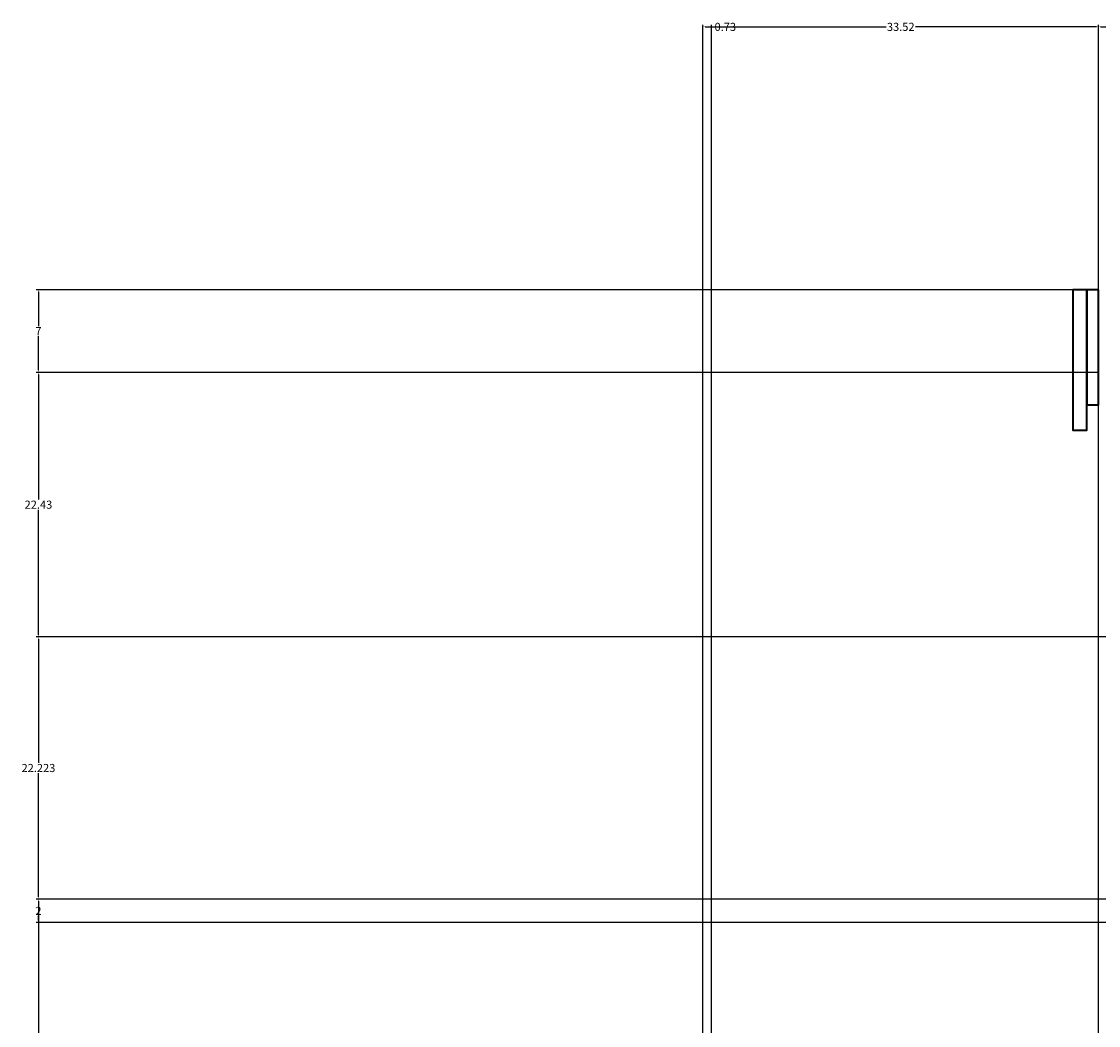
# Model space of a CAD drawing. Units: inches. Extents: x -139 to 346, y 72 to 413.
# Tile 6 of 18: x -139 to -47, y 328 to 413. Entities that reach past the tile are written whole.
import ezdxf

# ---------------------------------------------------------------- set-up
doc = ezdxf.new("R2010")
doc.units = ezdxf.units.IN
doc.header["$MEASUREMENT"] = 0
doc.layers.add('A-ANNO-DIMS', color=2, linetype='Continuous', lineweight=18)
doc.layers.add('A-ROOF', color=1, linetype='Continuous', lineweight=35)
doc.styles.get("Standard").update_dxf_attribs({"font": 'arial.ttf'})
doc.dimstyles.get("Standard").update_dxf_attribs({"dimtxt": 0.6875, "dimasz": 0.18, "dimexe": 0.18, "dimexo": 0.0625, "dimgap": 0.09, "dimtad": 0, "dimtih": 1, "dimtoh": 1, "dimdec": 4, "dimzin": 0, "dimdsep": 46, "dimlunit": 4, "dimtxsty": 'Standard', "dimcen": 0.09, "dimadec": 0, "dimazin": 0, "dimtfac": 1, "dimtdec": 4, "dimtofl": 0, "dimtmove": 0, "dimatfit": 3, "dimfxl": 1, "dimtolj": 1, "dimtzin": 0, "dimarcsym": 0})

# ---------------------------------------------------------------- blocks, each defined once
blk = doc.blocks.new('*D23')
at = {"layer": 'A-ANNO-DIMS', "color": 0, "lineweight": -2, "transparency": 16777216}
for p, q in [((-47.273, 383.037), (-47.273, 412.455)), ((-47.093, 412.275), (-22.053, 412.275)), ((5.493, 412.275), (-19.548, 412.275)), ((5.673, 338.384), (5.673, 412.455))]:
    blk.add_line(p, q, dxfattribs=at)
at = {"layer": 'A-ANNO-DIMS', "color": 0, "transparency": 16777216}
for points in [[(-47.093, 412.305), (-47.093, 412.245), (-47.273, 412.275)], [(5.493, 412.305), (5.493, 412.245), (5.673, 412.275)]]:
    blk.add_solid(points, dxfattribs=at)
at = {"layer": 'Defpoints', "color": 0, "transparency": 16777216}
for p in [(5.673, 412.275), (-47.273, 382.975), (5.673, 338.322)]:
    blk.add_point(p, dxfattribs=at)
at = {"layer": 'A-ANNO-DIMS', "color": 0, "transparency": 16777216, "insert": (-20.8, 412.275), "char_height": 0.6875, "attachment_point": 5}
blk.add_mtext('\\A1;52.95', dxfattribs=at)
blk = doc.blocks.new('*D44')
at = {"layer": 'A-ANNO-DIMS', "color": 0, "lineweight": -2, "transparency": 16777216}
for p, q in [((5.61, 338.322), (-137.304, 338.322)), ((-137.124, 338.142), (-137.124, 315.132)), ((-137.124, 291.24), (-137.124, 314.25)), ((-47.336, 291.06), (-137.304, 291.06))]:
    blk.add_line(p, q, dxfattribs=at)
at = {"layer": 'A-ANNO-DIMS', "color": 0, "transparency": 16777216}
for points in [[(-137.154, 338.142), (-137.094, 338.142), (-137.124, 338.322)], [(-137.154, 291.24), (-137.094, 291.24), (-137.124, 291.06)]]:
    blk.add_solid(points, dxfattribs=at)
at = {"layer": 'Defpoints', "color": 0, "transparency": 16777216}
for p in [(-137.124, 338.322), (5.673, 338.322), (-47.273, 291.06)]:
    blk.add_point(p, dxfattribs=at)
at = {"layer": 'A-ANNO-DIMS', "color": 0, "transparency": 16777216, "insert": (-137.124, 314.691), "char_height": 0.6875, "attachment_point": 5}
blk.add_mtext('\\A1;47.26', dxfattribs=at)
blk = doc.blocks.new('*D45')
at = {"layer": 'A-ANNO-DIMS', "color": 0, "lineweight": -2, "transparency": 16777216}
for p, q in [((-34.797, 360.544), (-137.304, 360.544)), ((-137.124, 360.364), (-137.124, 349.874)), ((-137.124, 338.502), (-137.124, 348.992)), ((5.61, 338.322), (-137.304, 338.322))]:
    blk.add_line(p, q, dxfattribs=at)
at = {"layer": 'A-ANNO-DIMS', "color": 0, "transparency": 16777216}
for points in [[(-137.154, 360.364), (-137.094, 360.364), (-137.124, 360.544)], [(-137.154, 338.502), (-137.094, 338.502), (-137.124, 338.322)]]:
    blk.add_solid(points, dxfattribs=at)
at = {"layer": 'Defpoints', "color": 0, "transparency": 16777216}
for p in [(-137.124, 360.544), (-34.735, 360.544), (5.673, 338.322)]:
    blk.add_point(p, dxfattribs=at)
at = {"layer": 'A-ANNO-DIMS', "color": 0, "transparency": 16777216, "insert": (-137.124, 349.433), "char_height": 0.6875, "attachment_point": 5}
blk.add_mtext('\\A1;22.223', dxfattribs=at)
blk = doc.blocks.new('*D46')
at = {"layer": 'A-ANNO-DIMS', "color": 0, "lineweight": -2, "transparency": 16777216}
for p, q in [((-47.336, 382.975), (-137.304, 382.975)), ((-137.124, 382.795), (-137.124, 372.201)), ((-137.124, 360.724), (-137.124, 371.318)), ((-34.797, 360.544), (-137.304, 360.544))]:
    blk.add_line(p, q, dxfattribs=at)
at = {"layer": 'A-ANNO-DIMS', "color": 0, "transparency": 16777216}
for points in [[(-137.154, 382.795), (-137.094, 382.795), (-137.124, 382.975)], [(-137.154, 360.724), (-137.094, 360.724), (-137.124, 360.544)]]:
    blk.add_solid(points, dxfattribs=at)
at = {"layer": 'Defpoints', "color": 0, "transparency": 16777216}
for p in [(-137.124, 382.975), (-47.273, 382.975), (-34.735, 360.544)]:
    blk.add_point(p, dxfattribs=at)
at = {"layer": 'A-ANNO-DIMS', "color": 0, "transparency": 16777216, "insert": (-137.124, 371.76), "char_height": 0.6875, "attachment_point": 5}
blk.add_mtext('\\A1;22.43', dxfattribs=at)
blk = doc.blocks.new('*D47')
at = {"layer": 'A-ANNO-DIMS', "color": 0, "lineweight": -2, "transparency": 16777216}
for p, q in [((-47.335936, 389.974785), (-137.303687, 389.974785)), ((-137.123687, 389.794785), (-137.123687, 386.908535)), ((-137.123687, 383.154785), (-137.123687, 386.041035)), ((-47.335936, 382.974785), (-137.303687, 382.974785))]:
    blk.add_line(p, q, dxfattribs=at)
at = {"layer": 'A-ANNO-DIMS', "color": 0, "transparency": 16777216}
for points in [[(-137.153687, 389.794785), (-137.093687, 389.794785), (-137.123687, 389.974785)], [(-137.153687, 383.154785), (-137.093687, 383.154785), (-137.123687, 382.974785)]]:
    blk.add_solid(points, dxfattribs=at)
at = {"layer": 'Defpoints', "color": 0, "transparency": 16777216}
for p in [(-137.123687, 389.974785), (-47.273436, 389.974785), (-47.273436, 382.974785)]:
    blk.add_point(p, dxfattribs=at)
at = {"layer": 'A-ANNO-DIMS', "color": 0, "transparency": 16777216, "insert": (-137.123687, 386.474785), "char_height": 0.6875, "attachment_point": 5}
blk.add_mtext('\\A1;7', dxfattribs=at)
blk = doc.blocks.new('*D49')
at = {"layer": 'A-ANNO-DIMS', "color": 0, "lineweight": -2, "transparency": 16777216}
for p, q in [((-80.796, 213.573), (-80.796, 412.455)), ((-80.616, 412.275), (-65.281, 412.275)), ((-47.453, 412.275), (-62.789, 412.275)), ((-47.273, 226.669), (-47.273, 412.455))]:
    blk.add_line(p, q, dxfattribs=at)
at = {"layer": 'A-ANNO-DIMS', "color": 0, "transparency": 16777216}
for points in [[(-80.616, 412.305), (-80.616, 412.245), (-80.796, 412.275)], [(-47.453, 412.305), (-47.453, 412.245), (-47.273, 412.275)]]:
    blk.add_solid(points, dxfattribs=at)
at = {"layer": 'Defpoints', "color": 0, "transparency": 16777216}
for p in [(-47.273, 412.275), (-47.273, 226.606), (-80.796, 213.511)]:
    blk.add_point(p, dxfattribs=at)
at = {"layer": 'A-ANNO-DIMS', "color": 0, "transparency": 16777216, "insert": (-64.035, 412.275), "char_height": 0.6875, "attachment_point": 5}
blk.add_mtext('\\A1;33.52', dxfattribs=at)
blk = doc.blocks.new('*D50')
at = {"layer": 'A-ANNO-DIMS', "color": 0, "lineweight": -2, "transparency": 16777216}
for p, q in [((-80.796, 213.573), (-80.796, 412.455)), ((-80.616, 412.275), (-80.248, 412.275)), ((-80.068, 211.71), (-80.068, 412.455)), ((-80.068, 412.275), (-79.888, 412.275))]:
    blk.add_line(p, q, dxfattribs=at)
at = {"layer": 'A-ANNO-DIMS', "color": 0, "transparency": 16777216}
for points in [[(-80.616, 412.305), (-80.616, 412.245), (-80.796, 412.275)], [(-80.248, 412.305), (-80.248, 412.245), (-80.068, 412.275)]]:
    blk.add_solid(points, dxfattribs=at)
at = {"layer": 'Defpoints', "color": 0, "transparency": 16777216}
for p in [(-80.068, 412.275), (-80.796, 213.511), (-80.068, 211.648)]:
    blk.add_point(p, dxfattribs=at)
at = {"layer": 'A-ANNO-DIMS', "color": 0, "transparency": 16777216, "insert": (-78.905, 412.275), "char_height": 0.6875, "attachment_point": 5}
blk.add_mtext('\\A1;0.73', dxfattribs=at)
blk = doc.blocks.new('*D89')
at = {"layer": 'A-ANNO-DIMS', "color": 0, "lineweight": -2, "transparency": 16777216}
for p, q in [((62.363, 338.322), (-137.304, 338.322)), ((-137.124, 338.142), (-137.124, 315.132)), ((-137.124, 291.24), (-137.124, 314.25)), ((62.363, 291.06), (-137.304, 291.06))]:
    blk.add_line(p, q, dxfattribs=at)
at = {"layer": 'A-ANNO-DIMS', "color": 0, "transparency": 16777216}
for points in [[(-137.154, 338.142), (-137.094, 338.142), (-137.124, 338.322)], [(-137.154, 291.24), (-137.094, 291.24), (-137.124, 291.06)]]:
    blk.add_solid(points, dxfattribs=at)
at = {"layer": 'Defpoints', "color": 0, "transparency": 16777216}
for p in [(-137.124, 338.322), (62.426, 338.322), (62.426, 291.06)]:
    blk.add_point(p, dxfattribs=at)
at = {"layer": 'A-ANNO-DIMS', "color": 0, "transparency": 16777216, "insert": (-137.124, 314.691), "char_height": 0.6875, "attachment_point": 5}
blk.add_mtext('\\A1;47.26', dxfattribs=at)
blk = doc.blocks.new('*D92')
at = {"layer": 'A-ANNO-DIMS', "color": 0, "lineweight": -2, "transparency": 16777216}
for p, q in [((62.363, 338.322), (-137.304, 338.322)), ((-137.124, 338.142), (-137.124, 337.757)), ((-137.124, 336.502), (-137.124, 336.887)), ((60.363, 336.322), (-137.304, 336.322))]:
    blk.add_line(p, q, dxfattribs=at)
at = {"layer": 'A-ANNO-DIMS', "color": 0, "transparency": 16777216}
for points in [[(-137.154, 338.142), (-137.094, 338.142), (-137.124, 338.322)], [(-137.154, 336.502), (-137.094, 336.502), (-137.124, 336.322)]]:
    blk.add_solid(points, dxfattribs=at)
at = {"layer": 'Defpoints', "color": 0, "transparency": 16777216}
for p in [(62.426, 338.322), (-137.124, 336.322), (60.426, 336.322)]:
    blk.add_point(p, dxfattribs=at)
at = {"layer": 'A-ANNO-DIMS', "color": 0, "transparency": 16777216, "insert": (-137.124, 337.322), "char_height": 0.6875, "attachment_point": 5}
blk.add_mtext('\\A1;2', dxfattribs=at)

msp = doc.modelspace()

# ---------------------------------------------------------------- linework, layer by layer
at = {"layer": 'A-ROOF'}
for points in [[(-48.2494, 389.9748), (-49.454, 389.9748), (-49.454, 378.0862), (-48.2494, 378.0862)], [(-47.2734, 389.9748), (-48.2494, 389.9748), (-48.2494, 380.2199), (-47.2734, 380.2199)]]:
    msp.add_lwpolyline(points, close=True, dxfattribs=at)

# ---------------------------------------------------------------- dimensions: what is measured, and where the dimension line sits
at = {"layer": 'A-ANNO-DIMS'}
for base, p1, p2, picture, middle in [((-47.2734, 412.2748), (-80.7961, 213.5107), (-47.2734, 226.6062), '*D49', (-64.0348, 412.2748)), ((-80.0684, 412.2748), (-80.7961, 213.5107), (-80.0684, 211.6478), '*D50', (-78.9055, 412.2748)), ((5.6729, 412.2748), (-47.2734, 382.9748), (5.6729, 338.3217), '*D23', (-20.8002, 412.2748))]:
    dim = msp.add_linear_dim(base=base, p1=p1, p2=p2, dimstyle='Standard', override={"dimdec": 2, "dimlfac": 1, "dimrnd": 0, "dimzin": 0, "dimdsep": 46, "dimlunit": 2}, dxfattribs=at)
    dim.commit()
    dim.dimension.update_dxf_attribs({"geometry": picture, "text_midpoint": middle})
for base, p1, p2, override, picture, middle in [((-137.1237, 389.9748), (-47.2734, 382.9748), (-47.2734, 389.9748), {"dimdec": 0, "dimlfac": 1, "dimrnd": 0, "dimzin": 0, "dimdsep": 46, "dimlunit": 2}, '*D47', (-137.1237, 386.4748)), ((-137.1237, 382.9748), (-34.7346, 360.5443), (-47.2734, 382.9748), {"dimdec": 2, "dimlfac": 1, "dimrnd": 0, "dimzin": 0, "dimdsep": 46, "dimlunit": 2}, '*D46', (-137.1237, 371.7595)), ((-137.1237, 360.5443), (5.6729, 338.3217), (-34.7346, 360.5443), {"dimdec": 3, "dimlfac": 1, "dimrnd": 0, "dimzin": 0, "dimdsep": 46, "dimlunit": 2}, '*D45', (-137.1237, 349.433)), ((-137.1237, 338.3217), (-47.2734, 291.0604), (5.6729, 338.3217), {"dimdec": 2, "dimlfac": 1, "dimrnd": 0, "dimzin": 0, "dimdsep": 46, "dimlunit": 2}, '*D44', (-137.1237, 314.691)), ((-137.1237, 338.3217), (62.4258, 291.0604), (62.4258, 338.3217), {"dimdec": 2, "dimlfac": 1, "dimrnd": 0, "dimzin": 0, "dimdsep": 46, "dimlunit": 2}, '*D89', (-137.1237, 314.691)), ((-137.1237, 336.3217), (62.4258, 338.3217), (60.4258, 336.3217), {"dimdec": 0, "dimlfac": 1, "dimrnd": 0, "dimzin": 0, "dimdsep": 46, "dimlunit": 2}, '*D92', (-137.1237, 337.3217))]:
    dim = msp.add_linear_dim(base=base, p1=p1, p2=p2, angle=90, dimstyle='Standard', override=override, dxfattribs=at)
    dim.commit()
    dim.dimension.update_dxf_attribs({"geometry": picture, "text_midpoint": middle})

doc.saveas('drawing.dxf')
